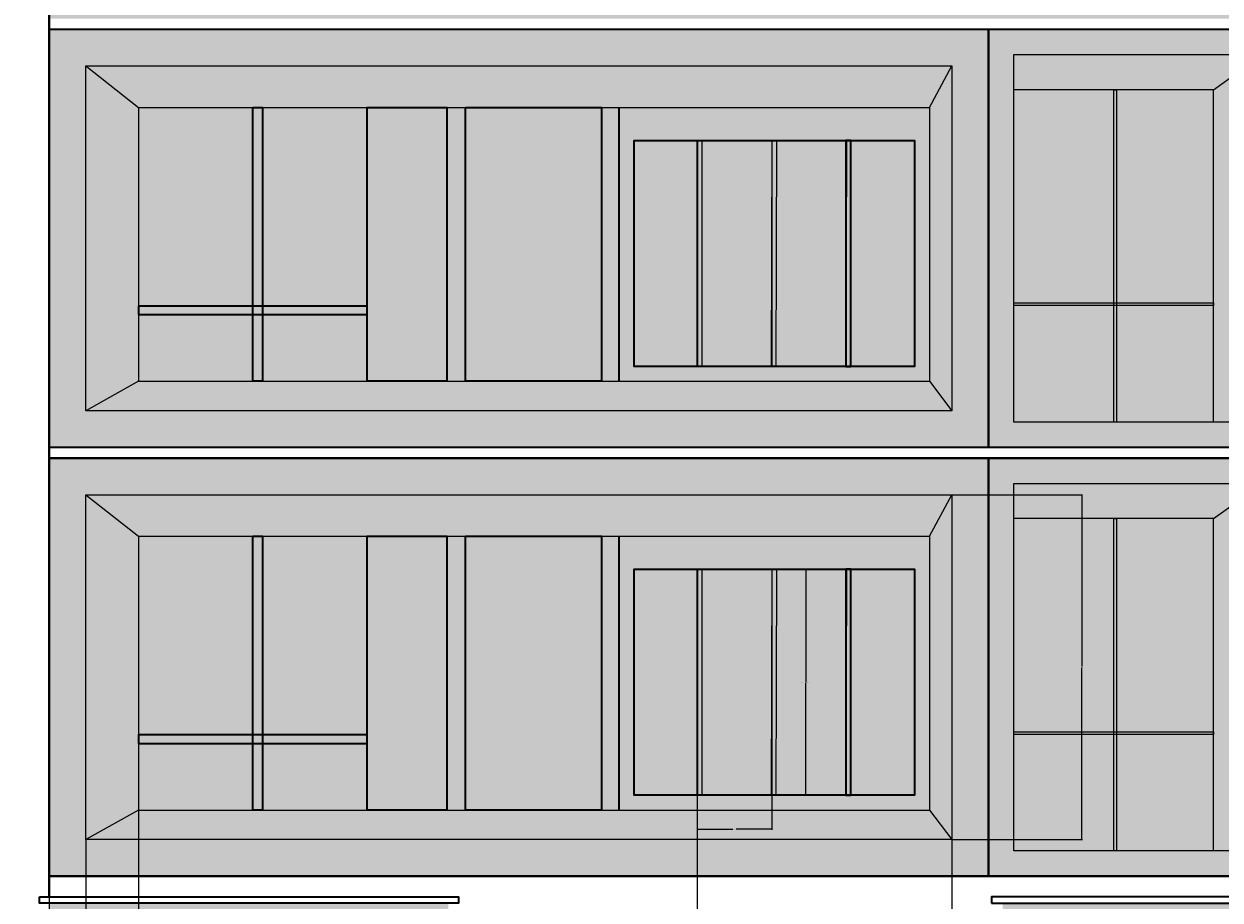
# Model space of a CAD drawing. Units: feet. Extents: x 1141 to 2858, y 751 to 1654.
# Tile 3 of 13: x 1718 to 2096, y 918 to 1195. Entities that reach past the tile are written whole.
import ezdxf

# ---------------------------------------------------------------- set-up
doc = ezdxf.new("R2010")
doc.units = ezdxf.units.FT
for name, color, linetype, lineweight in [('A-ANNO-DIMS', 2, 'Continuous', 18), ('A-ELEV', 7, 'Continuous', 35), ('A-ELEV-PATT', 8, 'Continuous', 13), ('A-GLAZ', 4, 'Continuous', 25)]:
    doc.layers.add(name, color=color, linetype=linetype, lineweight=lineweight)
doc.styles.get("Standard").update_dxf_attribs({"font": 'arial.ttf'})
doc.dimstyles.get("Standard").update_dxf_attribs({"dimtxt": 0.18, "dimasz": 0.18, "dimexe": 0.18, "dimexo": 0.0625, "dimgap": 0.09, "dimtad": 0, "dimtih": 1, "dimtoh": 1, "dimdec": 1, "dimzin": 0, "dimdsep": 46, "dimlunit": 3, "dimtxsty": 'Standard', "dimcen": 0.09, "dimadec": 0, "dimazin": 0, "dimtfac": 1, "dimtdec": 1, "dimtofl": 0, "dimtmove": 0, "dimatfit": 3, "dimfxl": 1, "dimtolj": 1, "dimtzin": 0, "dimarcsym": 0})

# ---------------------------------------------------------------- blocks, each defined once
blk = doc.blocks.new('WIN-SIDE-A')
blk.add_line((63.09, 104.94), (78.57, 116.03))
blk.add_line((63.09, 104.94), (78.57, 116.03))
for points in [[(78.57, 0), (0, 0), (0, 116.03), (78.57, 116.03)], [(78.57, 0), (0, 0), (0, 116.03), (78.57, 116.03)], [(31.54, 104.94), (32.46, 104.94), (32.46, 0), (31.54, 0)], [(0, 37.61), (63.09, 37.61), (63.09, 36.79), (0, 36.79)]]:
    blk.add_lwpolyline(points, close=True)
for points in [[(63.09, 0), (63.09, 104.94), (0, 104.94)], [(63.09, 0), (63.09, 104.94), (0, 104.94)], [(31.54, 37.61), (31.54, 104.94), (32.46, 104.94), (32.46, 37.61)], [(31.54, 36.79), (0, 36.79), (0, 37.61), (31.54, 37.61)], [(32.46, 36.79), (32.46, 0), (31.54, 0), (31.54, 36.79)], [(32.46, 37.61), (63.09, 37.61), (63.09, 36.79), (32.46, 36.79)]]:
    blk.add_lwpolyline(points)
blk = doc.blocks.new('BALCONY-GLAZ-A')
for p, q in [((0, 108.84), (16.63, 95.74)), ((0, 108.84), (16.63, 95.74)), ((266.62, 95.74), (273.67, 108.84)), ((266.62, 95.74), (273.67, 108.84)), ((16.63, 95.74), (16.63, 9.29)), ((16.63, 95.74), (266.62, 95.74)), ((16.63, 95.74), (16.63, 9.29)), ((16.63, 95.74), (266.62, 95.74)), ((266.62, 95.74), (266.62, 9.19)), ((266.62, 95.74), (266.62, 9.19)), ((16.63, 9.29), (0, 0)), ((16.63, 9.29), (0, 0)), ((16.63, 9.29), (266.62, 9.29)), ((16.63, 9.29), (266.62, 9.29)), ((266.62, 9.29), (273.67, 0)), ((266.62, 9.29), (273.67, 0))]:
    blk.add_line(p, q)
for points in [[(0, 108.84), (273.67, 108.84), (273.67, 0), (0, 0)], [(0, 108.84), (273.67, 108.84), (273.67, 0), (0, 0)], [(266.62, 9.19), (168.47, 9.19), (168.47, 95.74), (266.62, 95.74)], [(266.62, 9.19), (168.47, 9.19), (168.47, 95.74), (266.62, 95.74)]]:
    blk.add_lwpolyline(points, close=True)
blk = doc.blocks.new('WIN-SLIDING')
for points in [[(36.16, 23.71), (36.16, 86.44), (39.2, 86.44), (39.2, 23.71)], [(36.16, 23.71), (0, 23.71), (0, 21.05), (36.16, 21.05)], [(39.2, 21.05), (72.32, 21.05), (72.32, 23.71), (39.2, 23.71)], [(39.2, 21.05), (39.2, 0), (36.16, 0), (36.16, 21.05)]]:
    blk.add_lwpolyline(points)
blk = doc.blocks.new('GLAZ-PANEL-A')
blk.add_lwpolyline([(1.57, 71.37), (0, 71.37), (0, 0), (1.57, 0)], close=True)
for points in [[(1.57, 71.37), (23.57, 71.37)], [(1.57, 0), (1.57, 71.37)], [(23.57, 71.37), (23.57, 0)], [(23.57, 0), (1.57, 0)]]:
    blk.add_lwpolyline(points)
blk = doc.blocks.new('*D10')
at = {"layer": 'A-ANNO-DIMS', "color": 0, "lineweight": -2, "transparency": 16777216}
for p, q in [((1954.44, 1022.8), (1965.26, 1022.8)), ((1965.08, 1022.62), (1965.08, 987.3)), ((1965.08, 951.61), (1965.08, 986.93)), ((1954.44, 951.43), (1965.26, 951.43))]:
    blk.add_line(p, q, dxfattribs=at)
at = {"layer": 'A-ANNO-DIMS', "color": 0, "transparency": 16777216}
for points in [[(1965.05, 1022.62), (1965.11, 1022.62), (1965.08, 1022.8)], [(1965.05, 951.61), (1965.11, 951.61), (1965.08, 951.43)]]:
    blk.add_solid(points, dxfattribs=at)
at = {"layer": 'Defpoints', "color": 0, "transparency": 16777216}
for p in [(1954.37, 1022.8), (1965.08, 1022.8), (1954.37, 951.43)]:
    blk.add_point(p, dxfattribs=at)
at = {"layer": 'A-ANNO-DIMS', "color": 0, "transparency": 16777216, "insert": (1965.08, 987.11), "char_height": 0.18, "attachment_point": 5}
blk.add_mtext('\\A1;GLAZING PANEL A 71 TYP.', dxfattribs=at)
blk = doc.blocks.new('*D11')
at = {"layer": 'A-ANNO-DIMS', "color": 0, "lineweight": -2, "transparency": 16777216}
for p, q in [((1930.8, 951.37), (1930.8, 940.54)), ((1954.37, 951.37), (1954.37, 940.54)), ((1930.98, 940.72), (1942.06, 940.72)), ((1954.19, 940.72), (1943.12, 940.72))]:
    blk.add_line(p, q, dxfattribs=at)
at = {"layer": 'A-ANNO-DIMS', "color": 0, "transparency": 16777216}
for points in [[(1930.98, 940.75), (1930.98, 940.69), (1930.8, 940.72)], [(1954.19, 940.75), (1954.19, 940.69), (1954.37, 940.72)]]:
    blk.add_solid(points, dxfattribs=at)
at = {"layer": 'Defpoints', "color": 0, "transparency": 16777216}
for p in [(1930.8, 951.43), (1954.37, 951.43), (1954.37, 940.72)]:
    blk.add_point(p, dxfattribs=at)
at = {"layer": 'A-ANNO-DIMS', "color": 0, "transparency": 16777216, "insert": (1942.59, 940.72), "char_height": 0.18, "attachment_point": 5}
blk.add_mtext('\\A1;24 TYP.', dxfattribs=at)
blk = doc.blocks.new('*D18')
at = {"layer": 'A-ANNO-DIMS', "color": 0, "lineweight": -2, "transparency": 16777216}
for p, q in [((1737.61, 937.42), (1737.61, 896.25)), ((2011.29, 937.42), (2011.29, 896.25)), ((1737.79, 896.43), (1872.51, 896.43)), ((2011.11, 896.43), (1876.38, 896.43))]:
    blk.add_line(p, q, dxfattribs=at)
at = {"layer": 'A-ANNO-DIMS', "color": 0, "transparency": 16777216}
for points in [[(1737.79, 896.46), (1737.79, 896.4), (1737.61, 896.43)], [(2011.11, 896.46), (2011.11, 896.4), (2011.29, 896.43)]]:
    blk.add_solid(points, dxfattribs=at)
at = {"layer": 'Defpoints', "color": 0, "transparency": 16777216}
for p in [(1737.61, 937.48), (2011.29, 937.48), (2011.29, 896.43)]:
    blk.add_point(p, dxfattribs=at)
at = {"layer": 'A-ANNO-DIMS', "color": 0, "transparency": 16777216, "insert": (1874.45, 896.43), "char_height": 0.18, "attachment_point": 5}
blk.add_mtext('\\A1;BALCONY GLAZING A 274 TYP.', dxfattribs=at)
blk = doc.blocks.new('*D19')
at = {"layer": 'A-ANNO-DIMS', "color": 0, "lineweight": -2, "transparency": 16777216}
for p, q in [((2011.35, 1046.32), (2052.52, 1046.32)), ((2052.34, 1046.14), (2052.34, 992.08)), ((2052.34, 937.66), (2052.34, 991.72)), ((2011.35, 937.48), (2052.52, 937.48))]:
    blk.add_line(p, q, dxfattribs=at)
at = {"layer": 'A-ANNO-DIMS', "color": 0, "transparency": 16777216}
for points in [[(2052.31, 1046.14), (2052.37, 1046.14), (2052.34, 1046.32)], [(2052.31, 937.66), (2052.37, 937.66), (2052.34, 937.48)]]:
    blk.add_solid(points, dxfattribs=at)
at = {"layer": 'Defpoints', "color": 0, "transparency": 16777216}
for p in [(2011.29, 1046.32), (2052.34, 1046.32), (2011.29, 937.48)]:
    blk.add_point(p, dxfattribs=at)
at = {"layer": 'A-ANNO-DIMS', "color": 0, "transparency": 16777216, "insert": (2052.34, 991.9), "char_height": 0.18, "attachment_point": 5}
blk.add_mtext('\\A1;109 TYP.', dxfattribs=at)
blk = doc.blocks.new('*D24')
at = {"layer": 'A-ANNO-DIMS', "color": 0, "lineweight": -2, "transparency": 16777216}
for p, q in [((1725.97, 1599.45), (1668.14, 1599.45)), ((1668.32, 1599.27), (1668.32, 1202.86)), ((1668.32, 806.08), (1668.32, 1202.49)), ((1725.97, 805.9), (1668.14, 805.9))]:
    blk.add_line(p, q, dxfattribs=at)
at = {"layer": 'A-ANNO-DIMS', "color": 0, "transparency": 16777216}
for points in [[(1668.29, 1599.27), (1668.35, 1599.27), (1668.32, 1599.45)], [(1668.29, 806.08), (1668.35, 806.08), (1668.32, 805.9)]]:
    blk.add_solid(points, dxfattribs=at)
at = {"layer": 'Defpoints', "color": 0, "transparency": 16777216}
for p in [(1668.32, 1599.45), (1726.03, 1599.45), (1726.03, 805.9)]:
    blk.add_point(p, dxfattribs=at)
at = {"layer": 'A-ANNO-DIMS', "color": 0, "transparency": 16777216, "insert": (1668.32, 1202.68), "char_height": 0.18, "attachment_point": 5}
blk.add_mtext('\\A1;793.6', dxfattribs=at)
blk = doc.blocks.new('*D39')
at = {"layer": 'A-ANNO-DIMS', "color": 0, "lineweight": -2, "transparency": 16777216}
for p, q in [((2319.24, 1599.45), (1668.14, 1599.45)), ((1668.32, 1599.27), (1668.32, 1202.86)), ((1668.32, 806.08), (1668.32, 1202.49)), ((2319.24, 805.9), (1668.14, 805.9))]:
    blk.add_line(p, q, dxfattribs=at)
at = {"layer": 'A-ANNO-DIMS', "color": 0, "transparency": 16777216}
for points in [[(1668.29, 1599.27), (1668.35, 1599.27), (1668.32, 1599.45)], [(1668.29, 806.08), (1668.35, 806.08), (1668.32, 805.9)]]:
    blk.add_solid(points, dxfattribs=at)
at = {"layer": 'Defpoints', "color": 0, "transparency": 16777216}
for p in [(1668.32, 1599.45), (2319.3, 1599.45), (2319.3, 805.9)]:
    blk.add_point(p, dxfattribs=at)
at = {"layer": 'A-ANNO-DIMS', "color": 0, "transparency": 16777216, "insert": (1668.32, 1202.68), "char_height": 0.18, "attachment_point": 5}
blk.add_mtext('\\A1;793.6', dxfattribs=at)
blk = doc.blocks.new('*D89')
at = {"layer": 'A-ANNO-DIMS', "color": 0, "lineweight": -2, "transparency": 16777216}
for p, q in [((1754.24, 946.71), (1754.24, 751.07)), ((1726.03, 919.28), (1726.03, 751.07)), ((1726.21, 751.25), (1739.76, 751.25)), ((1754.06, 751.25), (1740.52, 751.25))]:
    blk.add_line(p, q, dxfattribs=at)
at = {"layer": 'A-ANNO-DIMS', "color": 0, "transparency": 16777216}
for points in [[(1726.21, 751.28), (1726.21, 751.22), (1726.03, 751.25)], [(1754.06, 751.28), (1754.06, 751.22), (1754.24, 751.25)]]:
    blk.add_solid(points, dxfattribs=at)
at = {"layer": 'Defpoints', "color": 0, "transparency": 16777216}
for p in [(1754.24, 946.77), (1726.03, 919.34), (1754.24, 751.25)]:
    blk.add_point(p, dxfattribs=at)
at = {"layer": 'A-ANNO-DIMS', "color": 0, "transparency": 16777216, "insert": (1740.14, 751.25), "char_height": 0.18, "attachment_point": 5}
blk.add_mtext('\\A1;28.21', dxfattribs=at)
blk = doc.blocks.new('*D90')
at = {"layer": 'A-ANNO-DIMS', "color": 0, "lineweight": -2, "transparency": 16777216}
for p, q in [((1930.8, 951.37), (1930.8, 751.07)), ((1726.03, 919.28), (1726.03, 751.07)), ((1726.21, 751.25), (1827.95, 751.25)), ((1930.62, 751.25), (1828.88, 751.25))]:
    blk.add_line(p, q, dxfattribs=at)
at = {"layer": 'A-ANNO-DIMS', "color": 0, "transparency": 16777216}
for points in [[(1726.21, 751.28), (1726.21, 751.22), (1726.03, 751.25)], [(1930.62, 751.28), (1930.62, 751.22), (1930.8, 751.25)]]:
    blk.add_solid(points, dxfattribs=at)
at = {"layer": 'Defpoints', "color": 0, "transparency": 16777216}
for p in [(1930.8, 951.43), (1726.03, 919.34), (1930.8, 751.25)]:
    blk.add_point(p, dxfattribs=at)
at = {"layer": 'A-ANNO-DIMS', "color": 0, "transparency": 16777216, "insert": (1828.42, 751.25), "char_height": 0.18, "attachment_point": 5}
blk.add_mtext('\\A1;204.77', dxfattribs=at)

msp = doc.modelspace()

# ---------------------------------------------------------------- hatches: boundary and pattern name
at = {"layer": 'A-ELEV-PATT'}
h = msp.add_hatch(color=256, dxfattribs=at)
h.dxf.hatch_style = 1
h.paths.add_polyline_path([(2206.032, 1599.4527), (2192.689, 1599.4527), (2192.689, 919.339), (2206.032, 919.339)])
h.paths.add_polyline_path([(2190.2416, 1599.4527), (2175.463, 1599.4527), (2175.463, 919.339), (2190.2416, 919.339)])
h.paths.add_polyline_path([(2173.0156, 1599.4527), (2117.407, 1599.4527), (2117.407, 919.339), (2173.0156, 919.339)])
h.paths.add_polyline_path([(2022.8666, 1057.9008), (1726.032, 1057.9008), (1726.032, 925.9008), (2022.8666, 925.9008)])
h.paths.add_polyline_path([(1737.6123, 937.4811), (1737.6123, 1046.3205), (2011.2863, 1046.3205), (2011.2863, 937.4811)], flags=16)
h.paths.add_polyline_path([(1754.2423, 946.7736), (1754.2423, 1033.2183), (2004.2323, 1033.2183), (2004.2323, 946.7736), (2004.3069, 946.6754), (1906.0824, 946.6754)], flags=0)
h.paths.add_polyline_path([(1900.5421, 946.7736), (1857.5566, 946.7736), (1857.5566, 1033.2183), (1900.5421, 1033.2183)], flags=0)
h.paths.add_polyline_path([(1910.8368, 951.4297), (1910.8368, 1022.7957), (1999.478, 1022.7957), (1999.478, 951.4297)], flags=0)
h.paths.add_polyline_path([(1930.8039, 951.4297), (1930.8039, 1022.7957), (1932.373, 1022.7957), (1932.373, 951.4297)], flags=0)
h.paths.add_polyline_path([(1851.6414, 946.7736), (1826.5664, 946.7736), (1826.5664, 967.8234), (1793.4402, 967.8234), (1793.4402, 946.7736), (1790.4043, 946.7736), (1790.4043, 967.8234), (1754.2423, 967.8234), (1754.2423, 970.4796), (1790.4043, 970.4796), (1790.4043, 1033.2183), (1793.4402, 1033.2183), (1793.4402, 970.4796), (1826.5664, 970.4796), (1826.5664, 1033.2183), (1851.6414, 1033.2183)], flags=0)
h.paths.add_polyline_path([(1954.3728, 951.4297), (1954.3728, 1022.7957), (1955.9419, 1022.7957), (1955.9419, 951.4297)], flags=0)
h.paths.add_polyline_path([(1977.7327, 951.4297), (1977.7327, 1022.7957), (1979.3018, 1022.7957), (1979.3018, 951.4297)], flags=0)
h.paths.add_polyline_path([(2022.8666, 1193.2888), (1726.032, 1193.2888), (1726.032, 1061.2888), (2022.8666, 1061.2888)])
h.paths.add_polyline_path([(1737.6123, 1072.869), (1737.6123, 1181.7085), (2011.2863, 1181.7085), (2011.2863, 1072.869)], flags=16)
h.paths.add_polyline_path([(1754.2423, 1082.1616), (1754.2423, 1168.6063), (2004.2323, 1168.6063), (2004.2323, 1082.1616), (2004.3069, 1082.0634), (1906.0824, 1082.0634)], flags=0)
h.paths.add_polyline_path([(1900.5421, 1082.1616), (1857.5566, 1082.1616), (1857.5566, 1168.6063), (1900.5421, 1168.6063)], flags=0)
h.paths.add_polyline_path([(1910.8368, 1086.8177), (1910.8368, 1158.1837), (1999.478, 1158.1837), (1999.478, 1086.8177)], flags=0)
h.paths.add_polyline_path([(1930.8039, 1086.8177), (1930.8039, 1158.1837), (1932.373, 1158.1837), (1932.373, 1086.8177)], flags=0)
h.paths.add_polyline_path([(1851.6414, 1082.1616), (1826.5664, 1082.1616), (1826.5664, 1103.2114), (1793.4402, 1103.2114), (1793.4402, 1082.1616), (1790.4043, 1082.1616), (1790.4043, 1103.2114), (1754.2423, 1103.2114), (1754.2423, 1105.8676), (1790.4043, 1105.8676), (1790.4043, 1168.6063), (1793.4402, 1168.6063), (1793.4402, 1105.8676), (1826.5664, 1105.8676), (1826.5664, 1168.6063), (1851.6414, 1168.6063)], flags=0)
h.paths.add_polyline_path([(1954.3728, 1086.8177), (1954.3728, 1158.1837), (1955.9419, 1158.1837), (1955.9419, 1086.8177)], flags=0)
h.paths.add_polyline_path([(1977.7327, 1086.8177), (1977.7327, 1158.1837), (1979.3018, 1158.1837), (1979.3018, 1086.8177)], flags=0)
h.paths.add_polyline_path([(2022.8666, 1599.4527), (1726.032, 1599.4527), (1726.032, 1467.4527), (2022.8666, 1467.4527)])
h.paths.add_polyline_path([(2011.2863, 1479.033), (1737.6123, 1479.033), (1737.6123, 1587.8725), (2011.2863, 1587.8725)], flags=16)
h.paths.add_polyline_path([(2004.2323, 1488.3255), (1754.2423, 1488.3255), (1754.2423, 1574.7702), (2004.2323, 1574.7702)], flags=0)
h.paths.add_polyline_path([(1829.1345, 1544.6458), (1914.1177, 1544.6458), (1914.1177, 1539.5463), (1830.9097, 1539.5463), (1831.6817, 1537.3286), (1914.1177, 1537.3286), (1914.1177, 1532.2291), (1833.4569, 1532.2291), (1834.229, 1530.0113), (1914.1177, 1530.0113), (1914.1177, 1524.9118), (1836.0042, 1524.9118), (1836.7762, 1522.694), (1914.1177, 1522.694), (1914.1177, 1517.5946), (1838.5514, 1517.5946), (1839.3235, 1515.3768), (1914.1177, 1515.3768), (1914.1177, 1510.2773), (1841.0987, 1510.2773), (1841.8707, 1508.0595), (1914.1177, 1508.0595), (1914.1177, 1502.9601), (1843.6459, 1502.9601), (1844.4179, 1500.7423), (1914.1177, 1500.7423), (1914.1177, 1495.6428), (1846.1931, 1495.6428), (1846.9652, 1493.425), (1914.1177, 1493.425), (1914.1177, 1488.3255), (1848.6593, 1488.3255), (1848.6593, 1488.5583)], flags=0)
h.paths.add_polyline_path([(2117.407, 1464.0647), (1820.5724, 1464.0647), (1820.5724, 1332.0647), (2117.407, 1332.0647)])
h.paths.add_polyline_path([(2105.8267, 1452.4845), (2105.8267, 1343.645), (1832.1527, 1343.645), (1832.1527, 1452.4845)], flags=16)
h.paths.add_polyline_path([(2089.1967, 1439.3822), (2089.1967, 1352.9376), (1937.3566, 1352.9376), (1937.3566, 1352.8393), (1839.1321, 1352.8393), (1839.2067, 1352.9376), (1839.2067, 1439.3822), (1937.3566, 1439.3822)], flags=0)
h.paths.add_polyline_path([(2016.8727, 1439.3822), (2016.8727, 1376.6436), (2049.9988, 1376.6436), (2049.9988, 1439.3822), (2053.0347, 1439.3822), (2053.0347, 1376.6436), (2089.1967, 1376.6436), (2089.1967, 1373.9873), (2053.0347, 1373.9873), (2053.0347, 1352.9376), (2049.9988, 1352.9376), (2049.9988, 1373.9873), (2016.8727, 1373.9873), (2016.8727, 1352.9376), (1991.7976, 1352.9376), (1991.7976, 1439.3822)], flags=0)
h.paths.add_polyline_path([(1985.8824, 1439.3822), (1985.8824, 1352.9376), (1942.8969, 1352.9376), (1942.8969, 1439.3822)], flags=0)
h.paths.add_polyline_path([(1932.6022, 1428.9596), (1932.6022, 1357.5937), (1843.961, 1357.5937), (1843.961, 1428.9596)], flags=0)
h.paths.add_polyline_path([(1912.6351, 1428.9596), (1912.6351, 1357.5937), (1911.066, 1357.5937), (1911.066, 1428.9596)], flags=0)
h.paths.add_polyline_path([(1889.0662, 1428.9596), (1889.0662, 1357.5937), (1887.4971, 1357.5937), (1887.4971, 1428.9596)], flags=0)
h.paths.add_polyline_path([(1865.7063, 1428.9596), (1865.7063, 1357.5937), (1864.1372, 1357.5937), (1864.1372, 1428.9596)], flags=0)
h.paths.add_polyline_path([(2117.407, 1328.6768), (1820.5724, 1328.6768), (1820.5724, 1196.6768), (2117.407, 1196.6768)])
h.paths.add_polyline_path([(2105.8267, 1317.0965), (2105.8267, 1208.257), (1832.1527, 1208.257), (1832.1527, 1317.0965)], flags=16)
h.paths.add_polyline_path([(2089.1967, 1303.9943), (2089.1967, 1217.5496), (1937.3566, 1217.5496), (1937.3566, 1217.4513), (1839.1321, 1217.4513), (1839.2067, 1217.5496), (1839.2067, 1303.9943), (1937.3566, 1303.9943)], flags=0)
h.paths.add_polyline_path([(2016.8727, 1303.9943), (2016.8727, 1241.2556), (2049.9988, 1241.2556), (2049.9988, 1303.9943), (2053.0347, 1303.9943), (2053.0347, 1241.2556), (2089.1967, 1241.2556), (2089.1967, 1238.5993), (2053.0347, 1238.5993), (2053.0347, 1217.5496), (2049.9988, 1217.5496), (2049.9988, 1238.5993), (2016.8727, 1238.5993), (2016.8727, 1217.5496), (1991.7976, 1217.5496), (1991.7976, 1303.9943)], flags=0)
h.paths.add_polyline_path([(1985.8824, 1303.9943), (1985.8824, 1217.5496), (1942.8969, 1217.5496), (1942.8969, 1303.9943)], flags=0)
h.paths.add_polyline_path([(1932.6022, 1293.5716), (1932.6022, 1222.2057), (1843.961, 1222.2057), (1843.961, 1293.5716)], flags=0)
h.paths.add_polyline_path([(1912.6351, 1293.5716), (1912.6351, 1222.2057), (1911.066, 1222.2057), (1911.066, 1293.5716)], flags=0)
h.paths.add_polyline_path([(1889.0662, 1293.5716), (1889.0662, 1222.2057), (1887.4971, 1222.2057), (1887.4971, 1293.5716)], flags=0)
h.paths.add_polyline_path([(1865.7063, 1293.5716), (1865.7063, 1222.2057), (1864.1372, 1222.2057), (1864.1372, 1293.5716)], flags=0)
h.paths.add_polyline_path([(2206.032, 917.3598), (2027.2589, 917.3598), (2027.2589, 805.9008), (2206.032, 805.9008)])
h.paths.add_polyline_path([(1852.1771, 917.3598), (1726.032, 917.3598), (1726.032, 805.9008), (1852.1771, 805.9008)])
h.paths.add_polyline_path([(2063.3101, 1580.3829), (2093.938, 1580.3829), (2093.938, 1513.0494), (2063.3101, 1513.0494)])
h.paths.add_polyline_path([(2063.3101, 1580.3829), (2093.938, 1580.3829), (2093.938, 1513.0494), (2063.3101, 1513.0494)])
h = msp.add_hatch(color=256, dxfattribs=at)
h.dxf.hatch_style = 1
h.paths.add_polyline_path([(2011.2863, 1587.8725), (1737.6123, 1587.8725), (1754.2423, 1574.7702), (2004.2323, 1574.7702)])
h.paths.add_polyline_path([(1754.2423, 1574.7702), (1737.6123, 1587.8725), (1737.6123, 1479.033), (1754.2423, 1488.3255)])
h.paths.add_polyline_path([(2011.2863, 1587.8725), (2004.2323, 1574.7702), (2004.2323, 1488.3255), (2011.2863, 1479.033)])
h.paths.add_polyline_path([(2004.2323, 1488.3255), (1754.2423, 1488.3255), (1737.6123, 1479.033), (2011.2863, 1479.033)])
h.paths.add_polyline_path([(2105.8267, 1452.4845), (1832.1527, 1452.4845), (1839.2067, 1439.3822), (1937.3566, 1439.3822), (2089.1967, 1439.3822)])
h.paths.add_polyline_path([(1839.2067, 1439.3822), (1832.1527, 1452.4845), (1832.1527, 1343.645), (1839.2067, 1352.9376)])
h.paths.add_polyline_path([(2105.8267, 1452.4845), (2089.1967, 1439.3822), (2089.1967, 1352.9376), (2105.8267, 1343.645)])
h.paths.add_polyline_path([(2089.1967, 1352.9376), (1937.3566, 1352.9376), (1937.3566, 1352.8393), (1839.1321, 1352.8393), (1832.1527, 1343.645), (2105.8267, 1343.645)])
h.paths.add_polyline_path([(1942.8969, 1439.3822), (1937.3566, 1439.3822), (1937.3566, 1352.9376), (1942.8969, 1352.9376)])
h.paths.add_polyline_path([(1991.7976, 1439.3822), (1985.8824, 1439.3822), (1985.8824, 1352.9376), (1991.7976, 1352.9376)])
h.paths.add_polyline_path([(2109.4211, 1591.4669), (2030.8524, 1591.4669), (2030.8524, 1580.3829), (2093.938, 1580.3829)])
h.paths.add_polyline_path([(2109.4211, 1591.4669), (2093.938, 1580.3829), (2093.938, 1475.4386), (2109.4211, 1475.4386)])
h.paths.add_polyline_path([(1991.7976, 1303.9943), (1985.8824, 1303.9943), (1985.8824, 1217.5496), (1991.7976, 1217.5496)])
h.paths.add_polyline_path([(1942.8969, 1303.9943), (1937.3566, 1303.9943), (1937.3566, 1217.5496), (1942.8969, 1217.5496)])
h.paths.add_polyline_path([(2105.8267, 1317.0965), (1832.1527, 1317.0965), (1839.2067, 1303.9943), (1937.3566, 1303.9943), (2089.1967, 1303.9943)])
h.paths.add_polyline_path([(1839.2067, 1303.9943), (1832.1527, 1317.0965), (1832.1527, 1208.257), (1839.2067, 1217.5496)])
h.paths.add_polyline_path([(2089.1967, 1217.5496), (1937.3566, 1217.5496), (1937.3566, 1217.4513), (1839.1321, 1217.4513), (1832.1527, 1208.257), (2105.8267, 1208.257)])
h.paths.add_polyline_path([(2105.8267, 1317.0965), (2089.1967, 1303.9943), (2089.1967, 1217.5496), (2105.8267, 1208.257)])
h.paths.add_polyline_path([(1754.2423, 1168.6063), (1737.6123, 1181.7085), (1737.6123, 1072.869), (1754.2423, 1082.1616)])
h.paths.add_polyline_path([(2011.2863, 1181.7085), (1737.6123, 1181.7085), (1754.2423, 1168.6063), (2004.2323, 1168.6063)])
h.paths.add_polyline_path([(2011.2863, 1181.7085), (2004.2323, 1168.6063), (2004.2323, 1082.1616), (2011.2863, 1072.869)])
h.paths.add_polyline_path([(2004.3069, 1082.0634), (1906.0824, 1082.0634), (1754.2423, 1082.1616), (1737.6123, 1072.869), (2011.2863, 1072.869)])
h.paths.add_polyline_path([(1906.0824, 1168.6063), (1900.5421, 1168.6063), (1900.5421, 1082.1616), (1906.0824, 1082.1616)])
h.paths.add_polyline_path([(1857.5566, 1168.6063), (1851.6414, 1168.6063), (1851.6414, 1082.1616), (1857.5566, 1082.1616)])
h.paths.add_polyline_path([(1906.0824, 1033.2183), (1900.5421, 1033.2183), (1900.5421, 946.7736), (1906.0824, 946.7736)])
h.paths.add_polyline_path([(1857.5566, 1033.2183), (1851.6414, 1033.2183), (1851.6414, 946.7736), (1857.5566, 946.7736)])
h.paths.add_polyline_path([(1754.2423, 1033.2183), (1737.6123, 1046.3205), (1737.6123, 937.4811), (1754.2423, 946.7736)])
h.paths.add_polyline_path([(2011.2863, 1046.3205), (1737.6123, 1046.3205), (1754.2423, 1033.2183), (2004.2323, 1033.2183)])
h.paths.add_polyline_path([(2011.2863, 1046.3205), (2004.2323, 1033.2183), (2004.2323, 946.7736), (2011.2863, 937.4811)])
h.paths.add_polyline_path([(2004.3069, 946.6754), (1906.0824, 946.6754), (1754.2423, 946.7736), (1737.6123, 937.4811), (2011.2863, 937.4811)])
h.paths.add_polyline_path([(2175.463, 1599.4527), (2173.0156, 1599.4527), (2173.0156, 919.339), (2175.463, 919.339)])
h = msp.add_hatch(color=256, dxfattribs=at)
h.dxf.hatch_style = 1
h.paths.add_polyline_path([(2062.3952, 1580.3829), (2030.8524, 1580.3829), (2030.8524, 1513.0494), (2062.3952, 1513.0494)])
h.paths.add_polyline_path([(2093.938, 1580.3829), (2063.3101, 1580.3829), (2063.3101, 1513.0494), (2093.938, 1513.0494)])
h.paths.add_polyline_path([(2093.938, 1512.23), (2063.3101, 1512.23), (2063.3101, 1475.4386), (2093.938, 1475.4386)])
h.paths.add_polyline_path([(2062.3952, 1512.23), (2030.8524, 1512.23), (2030.8524, 1475.4386), (2062.3952, 1475.4386)])
h.paths.add_polyline_path([(1780.1289, 1444.9949), (1749.501, 1444.9949), (1749.501, 1377.6615), (1780.1289, 1377.6615)])
h.paths.add_polyline_path([(1812.5866, 1444.9949), (1781.0438, 1444.9949), (1781.0438, 1377.6615), (1812.5866, 1377.6615)])
h.paths.add_polyline_path([(1812.5866, 1376.842), (1781.0438, 1376.842), (1781.0438, 1340.0506), (1812.5866, 1340.0506)])
h.paths.add_polyline_path([(1780.1289, 1376.842), (1749.501, 1376.842), (1749.501, 1340.0506), (1780.1289, 1340.0506)])
h.paths.add_polyline_path([(2105.8267, 1452.4845), (1832.1527, 1452.4845), (1832.1527, 1343.645), (1839.2067, 1352.9376), (1839.2067, 1439.3822), (1937.3566, 1439.3822), (1937.3566, 1352.9376), (1942.8969, 1352.9376), (1942.8969, 1439.3822), (1985.8824, 1439.3822), (1985.8824, 1352.9376), (1991.7976, 1352.9376), (1991.7976, 1439.3822), (2016.8727, 1439.3822), (2016.8727, 1376.6436), (2049.9988, 1376.6436), (2049.9988, 1439.3822), (2053.0347, 1439.3822), (2053.0347, 1376.6436), (2089.1967, 1376.6436), (2089.1967, 1373.9873), (2053.0347, 1373.9873), (2053.0347, 1352.9376), (2049.9988, 1352.9376), (1937.3566, 1352.9376), (1937.3566, 1352.8393), (1839.1321, 1352.8393), (1832.1527, 1343.645), (2105.8267, 1343.645)])
h.paths.add_polyline_path([(2049.9988, 1373.9873), (2016.8727, 1373.9873), (2016.8727, 1352.9376), (2049.9988, 1352.9376)], flags=17)
h.paths.add_polyline_path([(1780.1289, 1309.6069), (1749.501, 1309.6069), (1749.501, 1242.2735), (1780.1289, 1242.2735)])
h.paths.add_polyline_path([(1812.5866, 1309.6069), (1781.0438, 1309.6069), (1781.0438, 1242.2735), (1812.5866, 1242.2735)])
h.paths.add_polyline_path([(1812.5866, 1241.454), (1781.0438, 1241.454), (1781.0438, 1204.6626), (1812.5866, 1204.6626)])
h.paths.add_polyline_path([(1780.1289, 1241.454), (1749.501, 1241.454), (1749.501, 1204.6626), (1780.1289, 1204.6626)])
h.paths.add_polyline_path([(2049.9988, 1303.9943), (2016.8727, 1303.9943), (2016.8727, 1241.2556), (2049.9988, 1241.2556)])
h.paths.add_polyline_path([(2089.1967, 1303.9943), (2053.0347, 1303.9943), (2053.0347, 1241.2556), (2089.1967, 1241.2556)])
h.paths.add_polyline_path([(2089.1967, 1238.5993), (2053.0347, 1238.5993), (2053.0347, 1217.5496), (2089.1967, 1217.5496)])
h.paths.add_polyline_path([(2049.9988, 1238.5993), (2016.8727, 1238.5993), (2016.8727, 1217.5496), (2049.9988, 1217.5496)])
h.paths.add_polyline_path([(2062.3952, 1174.219), (2030.8524, 1174.219), (2030.8524, 1106.8855), (2062.3952, 1106.8855)])
h.paths.add_polyline_path([(2093.938, 1174.219), (2063.3101, 1174.219), (2063.3101, 1106.8855), (2093.938, 1106.8855)])
h.paths.add_polyline_path([(2093.938, 1106.066), (2063.3101, 1106.066), (2063.3101, 1069.2747), (2093.938, 1069.2747)])
h.paths.add_polyline_path([(2062.3952, 1106.066), (2030.8524, 1106.066), (2030.8524, 1069.2747), (2062.3952, 1069.2747)])
h.paths.add_polyline_path([(1906.0824, 1168.6063), (2004.2323, 1168.6063), (2011.2863, 1181.7085), (1737.6123, 1181.7085), (1737.6123, 1072.869), (2011.2863, 1072.869), (2004.3069, 1082.0634), (1906.0824, 1082.0634)])
h.paths.add_polyline_path([(1790.4043, 1168.6063), (1793.4402, 1168.6063), (1793.4402, 1105.8676), (1826.5664, 1105.8676), (1826.5664, 1168.6063), (1851.6414, 1168.6063), (1851.6414, 1082.1616), (1826.5664, 1082.1616), (1826.5664, 1103.2114), (1793.4402, 1103.2114), (1793.4402, 1082.1616), (1790.4043, 1082.1616), (1790.4043, 1103.2114), (1754.2423, 1103.2114), (1754.2423, 1105.8676), (1790.4043, 1105.8676)], flags=16)
h.paths.add_polyline_path([(1857.5566, 1168.6063), (1900.5421, 1168.6063), (1900.5421, 1082.1616), (1857.5566, 1082.1616)], flags=16)
h = msp.add_hatch(color=256, dxfattribs=at)
h.dxf.hatch_style = 1
h.paths.add_polyline_path([(1812.5866, 1456.0789), (1734.0179, 1456.0789), (1749.501, 1444.9949), (1812.5866, 1444.9949)], flags=0)
h.paths.add_polyline_path([(1820.5724, 1464.0647), (1726.032, 1464.0647), (1726.032, 1332.0647), (1820.5724, 1332.0647)])
h.paths.add_polyline_path([(1734.0179, 1456.0789), (1812.5866, 1456.0789), (1812.5866, 1340.0506), (1734.0179, 1340.0506)], flags=16)
h.paths.add_polyline_path([(1749.501, 1444.9949), (1781.0438, 1444.9949), (1781.0438, 1377.6615), (1812.5866, 1377.6615), (1812.5866, 1376.842), (1781.0438, 1376.842), (1781.0438, 1340.0506), (1780.1289, 1340.0506), (1780.1289, 1376.842), (1749.501, 1376.842), (1749.501, 1377.6615)], flags=0)
h.paths.add_polyline_path([(1749.501, 1444.9949), (1734.0179, 1456.0789), (1734.0179, 1340.0506), (1749.501, 1340.0506)], flags=0)
h.paths.add_polyline_path([(1820.5724, 1328.6768), (1726.032, 1328.6768), (1726.032, 1196.6768), (1820.5724, 1196.6768)])
h.paths.add_polyline_path([(1734.0179, 1320.6909), (1812.5866, 1320.6909), (1812.5866, 1204.6626), (1734.0179, 1204.6626)], flags=16)
h.paths.add_polyline_path([(1749.501, 1309.6069), (1781.0438, 1309.6069), (1781.0438, 1242.2735), (1812.5866, 1242.2735), (1812.5866, 1241.454), (1781.0438, 1241.454), (1781.0438, 1204.6626), (1780.1289, 1204.6626), (1780.1289, 1241.454), (1749.501, 1241.454), (1749.501, 1242.2735)], flags=0)
h.paths.add_polyline_path([(1749.501, 1309.6069), (1734.0179, 1320.6909), (1734.0179, 1204.6626), (1749.501, 1204.6626)], flags=0)
h.paths.add_polyline_path([(2117.407, 1193.2888), (2022.8666, 1193.2888), (2022.8666, 1061.2888), (2117.407, 1061.2888)])
h.paths.add_polyline_path([(2109.4211, 1185.3029), (2109.4211, 1069.2747), (2030.8524, 1069.2747), (2030.8524, 1185.3029)], flags=16)
h.paths.add_polyline_path([(2093.938, 1174.219), (2093.938, 1106.066), (2063.3101, 1106.066), (2063.3101, 1069.2747), (2062.3952, 1069.2747), (2062.3952, 1106.066), (2030.8524, 1106.066), (2030.8524, 1106.8855), (2062.3952, 1106.8855), (2062.3952, 1174.219), (2063.3101, 1174.219)], flags=0)
h.paths.add_polyline_path([(2702.6903, 1049.9149), (2624.1217, 1049.9149), (2624.1217, 1038.831), (2687.2072, 1038.831), (2687.2072, 933.8867), (2702.6903, 933.8867)], flags=0)
h.paths.add_polyline_path([(2109.4211, 1049.9149), (2093.938, 1038.831), (2093.938, 933.8867), (2109.4211, 933.8867)])
h.paths.add_polyline_path([(2109.4211, 1049.9149), (2030.8524, 1049.9149), (2030.8524, 1038.831), (2093.938, 1038.831)])
h = msp.add_hatch(color=256, dxfattribs=at)
h.dxf.hatch_style = 1
h.paths.add_polyline_path([(1219.3173, 1456.0789), (1140.7487, 1456.0789), (1156.2318, 1444.9949), (1219.3173, 1444.9949)], flags=0)
h.paths.add_polyline_path([(1156.2318, 1444.9949), (1140.7487, 1456.0789), (1140.7487, 1340.0506), (1156.2318, 1340.0506)], flags=0)
h.paths.add_polyline_path([(1156.2318, 1309.6069), (1187.7746, 1309.6069), (1187.7746, 1242.2735), (1219.3173, 1242.2735), (1219.3173, 1241.454), (1187.7746, 1241.454), (1187.7746, 1204.6626), (1186.8597, 1204.6626), (1186.8597, 1241.454), (1156.2318, 1241.454), (1156.2318, 1242.2735)], flags=0)
h.paths.add_polyline_path([(2109.4211, 1049.9149), (2030.8524, 1049.9149), (2030.8524, 1038.831), (2093.938, 1038.831), (2093.938, 933.8867), (2109.4211, 933.8867)], flags=0)
h.paths.add_polyline_path([(2109.4211, 1185.3029), (2030.8524, 1185.3029), (2030.8524, 1174.219), (2093.938, 1174.219), (2093.938, 1069.2747), (2109.4211, 1069.2747)])
h.paths.add_polyline_path([(1812.5866, 1320.6909), (1734.0179, 1320.6909), (1749.501, 1309.6069), (1812.5866, 1309.6069)])
h.paths.add_polyline_path([(1749.501, 1309.6069), (1734.0179, 1320.6909), (1734.0179, 1204.6626), (1749.501, 1204.6626)])
h.paths.add_polyline_path([(1812.5866, 1456.0789), (1734.0179, 1456.0789), (1749.501, 1444.9949), (1812.5866, 1444.9949)])
h.paths.add_polyline_path([(2117.407, 1057.9008), (2022.8666, 1057.9008), (2022.8666, 925.9008), (2117.407, 925.9008)])
h.paths.add_polyline_path([(2030.8524, 933.8867), (2030.8524, 1049.9149), (2109.4211, 1049.9149), (2109.4211, 933.8867)], flags=16)
h.paths.add_polyline_path([(2062.3952, 933.8867), (2062.3952, 970.6781), (2030.8524, 970.6781), (2030.8524, 971.4975), (2062.3952, 971.4975), (2062.3952, 1038.831), (2063.3101, 1038.831), (2093.938, 1038.831), (2093.938, 970.6781), (2063.3101, 970.6781), (2063.3101, 933.8867)], flags=0)
h = msp.add_hatch(color=256, dxfattribs=at)
h.dxf.hatch_style = 1
h.paths.add_polyline_path([(1512.5575, 1452.4845), (1238.8835, 1452.4845), (1238.8835, 1343.645), (1245.9375, 1352.9376), (1245.9375, 1439.3822), (1344.0874, 1439.3822), (1344.0874, 1352.9376), (1349.6277, 1352.9376), (1349.6277, 1439.3822), (1392.6132, 1439.3822), (1392.6132, 1352.9376), (1398.5284, 1352.9376), (1398.5284, 1439.3822), (1423.6034, 1439.3822), (1423.6034, 1376.6436), (1456.7296, 1376.6436), (1456.7296, 1439.3822), (1459.7654, 1439.3822), (1459.7654, 1376.6436), (1495.9275, 1376.6436), (1495.9275, 1373.9873), (1459.7654, 1373.9873), (1459.7654, 1352.9376), (1456.7296, 1352.9376), (1344.0874, 1352.9376), (1344.0874, 1352.8393), (1245.8629, 1352.8393), (1238.8835, 1343.645), (1512.5575, 1343.645)])
h.paths.add_polyline_path([(1790.4043, 1033.2183), (1754.2423, 1033.2183), (1754.2423, 970.4796), (1790.4043, 970.4796)])
h.paths.add_polyline_path([(1826.5664, 1033.2183), (1793.4402, 1033.2183), (1793.4402, 970.4796), (1826.5664, 970.4796)])
h.paths.add_polyline_path([(1826.5664, 967.8234), (1793.4402, 967.8234), (1793.4402, 946.7736), (1826.5664, 946.7736)])
h.paths.add_polyline_path([(1790.4043, 967.8234), (1754.2423, 967.8234), (1754.2423, 946.7736), (1790.4043, 946.7736)])
h.paths.add_polyline_path([(2093.938, 1038.831), (2063.3101, 1038.831), (2063.3101, 971.4975), (2093.938, 971.4975)])
h.paths.add_polyline_path([(2062.3952, 1038.831), (2030.8524, 1038.831), (2030.8524, 971.4975), (2062.3952, 971.4975)])
h.paths.add_polyline_path([(2062.3952, 970.6781), (2030.8524, 970.6781), (2030.8524, 933.8867), (2062.3952, 933.8867)])
h.paths.add_polyline_path([(2093.938, 970.6781), (2063.3101, 970.6781), (2063.3101, 933.8867), (2093.938, 933.8867)])
h = msp.add_hatch(color=256, dxfattribs=at)
h.dxf.hatch_style = 1
h.paths.add_polyline_path([(1985.8824, 1439.3822), (1942.8969, 1439.3822), (1942.8969, 1352.9376), (1985.8824, 1352.9376)])
h.paths.add_polyline_path([(1985.8824, 1303.9943), (1942.8969, 1303.9943), (1942.8969, 1217.5496), (1985.8824, 1217.5496)])
h.paths.add_polyline_path([(1900.5421, 1168.6063), (1857.5566, 1168.6063), (1857.5566, 1082.1616), (1900.5421, 1082.1616)])
h.paths.add_polyline_path([(1900.5421, 1033.2183), (1857.5566, 1033.2183), (1857.5566, 946.7736), (1900.5421, 946.7736)])
h = msp.add_hatch(color=256, dxfattribs=at)
h.dxf.hatch_style = 1
h.paths.add_polyline_path([(2030.7675, 1106.8895), (2062.3103, 1106.8895), (2062.3103, 1174.2229), (2063.2251, 1174.2229), (2063.2251, 1106.8895), (2093.8531, 1106.8895), (2093.8531, 1106.07), (2063.2251, 1106.07), (2063.2251, 1069.2786), (2062.3103, 1069.2786), (2062.3103, 1106.07), (2030.7675, 1106.07)])
h.paths.add_polyline_path([(1754.1574, 970.4836), (1790.3194, 970.4836), (1790.3194, 1033.2223), (1793.3553, 1033.2223), (1793.3553, 970.4836), (1826.4814, 970.4836), (1826.4814, 967.8273), (1793.3553, 967.8273), (1793.3553, 946.7776), (1790.3194, 946.7776), (1790.3194, 967.8273), (1754.1574, 967.8273)])
h.paths.add_polyline_path([(1905.9975, 1033.2223), (2004.1474, 1033.2223), (2004.1474, 946.7776), (1905.9975, 946.7776)])
h.paths.add_polyline_path([(1955.857, 1022.7996), (1955.857, 951.4337), (1977.6478, 951.4337), (1977.6478, 1022.7996)], flags=16)
h.paths.add_polyline_path([(1979.2168, 1022.7996), (1979.2168, 951.4337), (1999.393, 951.4337), (1999.393, 1022.7996)], flags=16)
h.paths.add_polyline_path([(1954.2879, 1022.7996), (1932.2881, 1022.7996), (1932.2881, 951.4337), (1954.2879, 951.4337)], flags=16)
h.paths.add_polyline_path([(1930.719, 1022.7996), (1910.7518, 1022.7996), (1910.7518, 951.4337), (1930.719, 951.4337)], flags=16)
h = msp.add_hatch(color=256, dxfattribs=at)
h.dxf.hatch_style = 1
h.paths.add_polyline_path([(1754.1574, 1105.8716), (1790.3194, 1105.8716), (1790.3194, 1168.6103), (1793.3553, 1168.6103), (1793.3553, 1105.8716), (1826.4814, 1105.8716), (1826.4814, 1103.2153), (1793.3553, 1103.2153), (1793.3553, 1082.1656), (1790.3194, 1082.1656), (1790.3194, 1103.2153), (1754.1574, 1103.2153)])
h.paths.add_polyline_path([(1905.9975, 1168.6103), (2004.1474, 1168.6103), (2004.1474, 1082.1656), (1905.9975, 1082.1656)])
h.paths.add_polyline_path([(1955.857, 1158.1876), (1955.857, 1086.8217), (1977.6478, 1086.8217), (1977.6478, 1158.1876)], flags=16)
h.paths.add_polyline_path([(1979.2168, 1158.1876), (1979.2168, 1086.8217), (1999.393, 1086.8217), (1999.393, 1158.1876)], flags=16)
h.paths.add_polyline_path([(1954.2879, 1158.1876), (1932.2881, 1158.1876), (1932.2881, 1086.8217), (1954.2879, 1086.8217)], flags=16)
h.paths.add_polyline_path([(1930.719, 1158.1876), (1910.7518, 1158.1876), (1910.7518, 1086.8217), (1930.719, 1086.8217)], flags=16)
h = msp.add_hatch(color=256, dxfattribs=at)
h.dxf.hatch_style = 1
h.paths.add_polyline_path([(1910.8932, 1157.9408), (1930.8603, 1157.9408), (1930.8603, 1086.5748), (1910.8932, 1086.5748)])
h.paths.add_polyline_path([(1979.3582, 1157.9408), (1999.5343, 1157.9408), (1999.5343, 1086.5748), (1979.3582, 1086.5748)])
h.paths.add_polyline_path([(1955.9983, 1157.9408), (1977.7891, 1157.9408), (1977.7891, 1086.5748), (1955.9983, 1086.5748)])
h.paths.add_polyline_path([(1932.4294, 1157.9408), (1954.4292, 1157.9408), (1954.4292, 1086.5748), (1932.4294, 1086.5748)])
h.paths.add_polyline_path([(1826.6227, 1168.3634), (1851.6978, 1168.3634), (1851.6978, 1081.9187), (1826.6227, 1081.9187)])
h = msp.add_hatch(color=256, dxfattribs=at)
h.dxf.hatch_style = 1
h.paths.add_polyline_path([(2030.7675, 971.5015), (2062.3103, 971.5015), (2062.3103, 1038.835), (2063.2251, 1038.835), (2063.2251, 971.5015), (2093.8531, 971.5015), (2093.8531, 970.682), (2063.2251, 970.682), (2063.2251, 933.8907), (2062.3103, 933.8907), (2062.3103, 970.682), (2030.7675, 970.682)])
h = msp.add_hatch(color=256, dxfattribs=at)
h.dxf.hatch_style = 1
h.paths.add_polyline_path([(1910.8932, 1022.5528), (1930.8603, 1022.5528), (1930.8603, 951.1869), (1910.8932, 951.1869)])
h.paths.add_polyline_path([(1979.3582, 1022.5528), (1999.5343, 1022.5528), (1999.5343, 951.1869), (1979.3582, 951.1869)])
h.paths.add_polyline_path([(1955.9983, 1022.5528), (1977.7891, 1022.5528), (1977.7891, 951.1869), (1955.9983, 951.1869)])
h.paths.add_polyline_path([(1932.4294, 1022.5528), (1954.4292, 1022.5528), (1954.4292, 951.1869), (1932.4294, 951.1869)])
h.paths.add_polyline_path([(1826.6227, 1032.9754), (1851.6978, 1032.9754), (1851.6978, 946.5307), (1826.6227, 946.5307)])

# ---------------------------------------------------------------- linework, layer by layer
at = {"layer": 'A-ELEV'}
for p, q in [((1726.032, 1599.4527), (1726.032, 919.339)), ((1726.032, 1599.4527), (1726.032, 919.339)), ((1726.032, 1079.009), (1726.032, 1199.009)), ((1726.032, 1079.009), (1726.032, 1199.009)), ((1726.032, 953.009), (1726.032, 1073.009)), ((1726.032, 953.009), (1726.032, 1073.009)), ((2117.407, 1057.9008), (1726.032, 1057.9008)), ((2117.407, 1057.9008), (1726.032, 1057.9008)), ((1726.032, 919.339), (1726.032, 947.009)), ((1726.032, 919.339), (1726.032, 947.009)), ((1726.032, 925.9008), (2117.407, 925.9008)), ((1726.032, 925.9008), (2117.407, 925.9008))]:
    msp.add_line(p, q, dxfattribs=at)
for points in [[(1726.032, 1193.2888), (2022.8666, 1193.2888), (2022.8666, 1061.2888), (1726.032, 1061.2888)], [(1726.032, 1193.2888), (2022.8666, 1193.2888), (2022.8666, 1061.2888), (1726.032, 1061.2888)], [(2117.407, 1061.2888), (2022.8666, 1061.2888), (2022.8666, 1193.2888), (2117.407, 1193.2888)], [(2117.407, 1061.2888), (2022.8666, 1061.2888), (2022.8666, 1193.2888), (2117.407, 1193.2888)], [(1790.4043, 1168.6063), (1793.4402, 1168.6063), (1793.4402, 1082.1616), (1790.4043, 1082.1616)], [(1851.6414, 1082.1616), (1826.5664, 1082.1616), (1826.5664, 1168.6063), (1851.6414, 1168.6063)], [(1851.6414, 1082.1616), (1826.5664, 1082.1616), (1826.5664, 1168.6063), (1851.6414, 1168.6063)], [(1857.5566, 1168.6063), (1900.5421, 1168.6063), (1900.5421, 1082.1616), (1857.5566, 1082.1616)], [(1857.5566, 1168.6063), (1900.5421, 1168.6063), (1900.5421, 1082.1616), (1857.5566, 1082.1616)], [(1999.478, 1086.8177), (1910.8368, 1086.8177), (1910.8368, 1158.1837), (1999.478, 1158.1837)], [(1979.3018, 1158.1837), (1977.7327, 1158.1837), (1977.7327, 1086.8177), (1979.3018, 1086.8177)], [(1754.2423, 1103.2114), (1826.5664, 1103.2114), (1826.5664, 1105.8676), (1754.2423, 1105.8676)], [(1726.032, 1057.9008), (2022.8666, 1057.9008), (2022.8666, 925.9008), (1726.032, 925.9008)], [(1726.032, 1057.9008), (2022.8666, 1057.9008), (2022.8666, 925.9008), (1726.032, 925.9008)], [(2117.407, 925.9008), (2022.8666, 925.9008), (2022.8666, 1057.9008), (2117.407, 1057.9008)], [(2117.407, 925.9008), (2022.8666, 925.9008), (2022.8666, 1057.9008), (2117.407, 1057.9008)], [(1790.4043, 1033.2183), (1793.4402, 1033.2183), (1793.4402, 946.7736), (1790.4043, 946.7736)], [(1851.6414, 946.7736), (1826.5664, 946.7736), (1826.5664, 1033.2183), (1851.6414, 1033.2183)], [(1851.6414, 946.7736), (1826.5664, 946.7736), (1826.5664, 1033.2183), (1851.6414, 1033.2183)], [(1857.5566, 1033.2183), (1900.5421, 1033.2183), (1900.5421, 946.7736), (1857.5566, 946.7736)], [(1857.5566, 1033.2183), (1900.5421, 1033.2183), (1900.5421, 946.7736), (1857.5566, 946.7736)], [(1999.478, 951.4297), (1910.8368, 951.4297), (1910.8368, 1022.7957), (1999.478, 1022.7957)], [(1979.3018, 1022.7957), (1977.7327, 1022.7957), (1977.7327, 951.4297), (1979.3018, 951.4297)], [(1754.2423, 967.8234), (1826.5664, 967.8234), (1826.5664, 970.4796), (1754.2423, 970.4796)], [(1722.9707, 919.339), (1855.3916, 919.339), (1855.3916, 917.3598), (1722.9707, 917.3598)], [(1722.9707, 919.339), (1855.3916, 919.339), (1855.3916, 917.3598), (1722.9707, 917.3598)], [(2023.7788, 917.3598), (2209.7297, 917.3598), (2209.7297, 919.339), (2023.7788, 919.339)], [(2023.7788, 917.3598), (2209.7297, 917.3598), (2209.7297, 919.339), (2023.7788, 919.339)]]:
    msp.add_lwpolyline(points, close=True, dxfattribs=at)
for points in [[(1906.0824, 1168.6063), (1906.0824, 1082.1616)], [(1906.0824, 1168.6063), (1906.0824, 1082.1616)], [(1930.8039, 1086.8177), (1910.8368, 1086.8177), (1910.8368, 1158.1837), (1930.8039, 1158.1837)], [(1930.8039, 1158.1837), (1930.8039, 1086.8177)], [(1979.3018, 1158.1837), (1999.478, 1158.1837), (1999.478, 1086.8177), (1979.3018, 1086.8177)], [(1979.3018, 1086.8177), (1979.3018, 1158.1837)], [(1906.0824, 1033.2183), (1906.0824, 946.7736)], [(1906.0824, 1033.2183), (1906.0824, 946.7736)], [(1930.8039, 951.4297), (1910.8368, 951.4297), (1910.8368, 1022.7957), (1930.8039, 1022.7957)], [(1930.8039, 1022.7957), (1930.8039, 951.4297)], [(1979.3018, 1022.7957), (1999.478, 1022.7957), (1999.478, 951.4297), (1979.3018, 951.4297)], [(1979.3018, 951.4297), (1979.3018, 1022.7957)]]:
    msp.add_lwpolyline(points, dxfattribs=at)

# ---------------------------------------------------------------- block references
at = {"layer": 'A-GLAZ'}
for name, p in [('WIN-SIDE-A', (2030.852, 1069.2751)), ('BALCONY-GLAZ-A', (1737.612, 1072.869)), ('WIN-SLIDING', (1754.242, 1082.162)), ('GLAZ-PANEL-A', (1930.804, 1086.818)), ('WIN-SIDE-A', (2030.852, 933.8871)), ('BALCONY-GLAZ-A', (1737.612, 937.481)), ('WIN-SLIDING', (1754.242, 946.774)), ('GLAZ-PANEL-A', (1930.804, 951.43))]:
    msp.add_blockref(name, p, dxfattribs=at)
at = {"layer": 'A-GLAZ', "rotation": 359.8141056446258}
for p in [(1954.1839, 1086.8445), (1954.1839, 951.4565)]:
    msp.add_blockref('GLAZ-PANEL-A', p, dxfattribs=at)

# ---------------------------------------------------------------- dimensions: what is measured, and where the dimension line sits
at = {"layer": 'A-ANNO-DIMS'}
for p1, p2, picture in [((1726.032, 805.9008), (1726.032, 1599.4527), '*D24'), ((2319.3013, 805.9008), (2319.3013, 1599.4527), '*D39')]:
    dim = msp.add_linear_dim(base=(1668.3207, 1599.4527), p1=p1, p2=p2, angle=90, dimstyle='Standard', override={"dimdec": 1, "dimlfac": 1, "dimrnd": 0, "dimzin": 0, "dimdsep": 46, "dimlunit": 2}, dxfattribs=at)
    dim.commit()
    dim.dimension.update_dxf_attribs({"geometry": picture, "text_midpoint": (1668.3207, 1202.6768)})
for base, p1, p2, text, picture, middle in [((2052.3374, 1046.3205), (2011.2863, 937.4811), (2011.2863, 1046.3205), '<> TYP.', '*D19', (2052.3374, 991.9008)), ((1965.0777, 1022.7957), (1954.3728, 951.4297), (1954.3728, 1022.7957), 'GLAZING PANEL A <> TYP.', '*D10', (1965.0777, 987.1127))]:
    dim = msp.add_linear_dim(base=base, p1=p1, p2=p2, angle=90, text=text, dimstyle='Standard', override={"dimdec": 0, "dimlfac": 1, "dimrnd": 0, "dimzin": 0, "dimdsep": 46, "dimlunit": 2}, dxfattribs=at)
    dim.commit()
    dim.dimension.update_dxf_attribs({"geometry": picture, "text_midpoint": middle})
for base, p2, picture, middle in [((1930.8039, 751.2508), (1930.8039, 951.4297), '*D90', (1828.418, 751.2508)), ((1754.2423, 751.2508), (1754.2423, 946.7736), '*D89', (1740.1372, 751.2508))]:
    dim = msp.add_linear_dim(base=base, p1=(1726.032, 919.339), p2=p2, dimstyle='Standard', override={"dimdec": 2, "dimlfac": 1, "dimrnd": 0, "dimzin": 0, "dimdsep": 46, "dimlunit": 2}, dxfattribs=at)
    dim.commit()
    dim.dimension.update_dxf_attribs({"geometry": picture, "text_midpoint": middle})
for base, p1, p2, text, picture, middle in [((1954.3728, 940.7248), (1930.8039, 951.4297), (1954.3728, 951.4297), '<> TYP.', '*D11', (1942.5884, 940.7248)), ((2011.2863, 896.43), (1737.6123, 937.4811), (2011.2863, 937.4811), 'BALCONY GLAZING A <> TYP.', '*D18', (1874.4493, 896.43))]:
    dim = msp.add_linear_dim(base=base, p1=p1, p2=p2, text=text, dimstyle='Standard', override={"dimdec": 0, "dimlfac": 1, "dimrnd": 0, "dimzin": 0, "dimdsep": 46, "dimlunit": 2}, dxfattribs=at)
    dim.commit()
    dim.dimension.update_dxf_attribs({"geometry": picture, "text_midpoint": middle})

doc.saveas('drawing.dxf')
